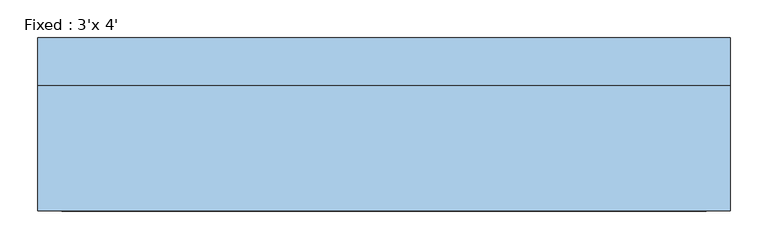
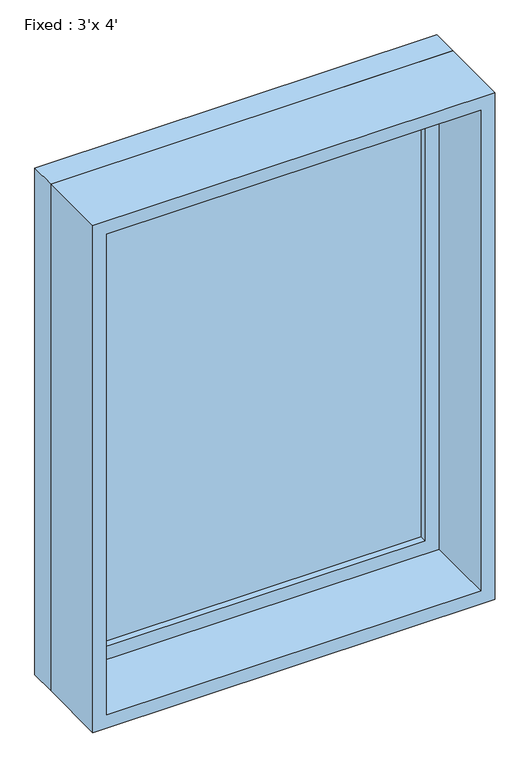
"""IFC4 building model written with IfcOpenShell, lengths in millimetres: window geometry, Fixed : 3'x 4'."""

from ifc_helpers import new_model, si_unit, frame, origin, place, context, project, spatial, polyline, outline, extrude, source, transform, mapped, element, save


def fixed_3_x_4_c1f32544(model_context):
    return source(origin(), model_context, "Body", "SweptSolid", [
        extrude(outline(polyline([(355.6, 66.675), (-431.8, 66.675), (-431.8, 79.375), (355.6, 79.375), (355.6, 66.675)])), frame((0.0, 0.0, 977.9), z_axis=(0.0, 0.0, 1.0), x_axis=(1.0, 0.0, 0.0)), (0.0, 0.0, 1.0), 1092.2),
        extrude(outline(polyline([(2114.55, -476.25), (933.45, -476.25), (933.45, 400.05), (2114.55, 400.05), (2114.55, -476.25)]), holes=[polyline([(2070.1, -431.8), (2070.1, 355.6), (977.9, 355.6), (977.9, -431.8), (2070.1, -431.8)])]), frame((0.0, 50.8, 0.0), z_axis=(0.0, 1.0, 0.0), x_axis=(0.0, 0.0, 1.0)), (0.0, 0.0, 1.0), 44.45),
        extrude(outline(polyline([(2133.6, -495.3), (914.4, -495.3), (914.4, 419.1), (2133.6, 419.1), (2133.6, -495.3)]), holes=[polyline([(2101.85, -463.55), (2101.85, 387.35), (946.15, 387.35), (946.15, -463.55), (2101.85, -463.55)])]), frame((0.0, -114.3, 0.0), z_axis=(0.0, 1.0, 0.0), x_axis=(0.0, 0.0, 1.0)), (0.0, 0.0, 1.0), 165.1),
        extrude(outline(polyline([(2133.6, 419.1), (2133.6, -495.3), (914.4, -495.3), (914.4, 419.1), (2133.6, 419.1)]), holes=[polyline([(2114.55, 400.05), (933.45, 400.05), (933.45, -476.25), (2114.55, -476.25), (2114.55, 400.05)])]), frame((0.0, 50.8, 0.0), z_axis=(0.0, 1.0, 0.0), x_axis=(0.0, 0.0, 1.0)), (0.0, 0.0, 1.0), 63.5),
    ])


if __name__ == "__main__":
    model = new_model("IFC4")
    model_context = context("Model", 3, world=origin())
    ifc_project = project(units=[si_unit("LENGTHUNIT", "METRE", prefix="MILLI")], contexts=[model_context])
    site = spatial("IfcSite", under=ifc_project)
    building = spatial("IfcBuilding", under=site)
    placement = place(None, origin())
    fixed_3_x_4_shape = fixed_3_x_4_c1f32544(model_context)
    element("IfcWindow", 1, ObjectType="Fixed : 3'x 4'", at=placement, inside=building, context=model_context, shape_type="MappedRepresentation", body=[
        mapped(fixed_3_x_4_shape, transform((0.0, 0.0, 0.0), x_axis=(1.0, 0.0, 0.0), y_axis=(0.0, 1.0, 0.0), z_axis=(0.0, 0.0, 1.0))),
    ])
    save(model, "model.ifc")

# Revit data of these elements
# Type "Fixed : 3'x 4'"
#   Type Mark = "18"
#   Construction Type Id = "GSP4R"
#   Assembly Code = "B2020100"
#   Analytic Construction = "1/8 in Pilkington single glazing"
#   Visual Light Transmittance = 0.9
#   Solar Heat Gain Coefficient = 0.78
#   Heat Transfer Coefficient (U) = 0.6496 BTU/(h·ft²·°F)
#   Height = 4' - 0"
#   Default Sill Height = 3' - 0"
#   Width = 3' - 0"
#   Window Inset = 0' - 0 3/4"
#   Define Thermal Properties by = 1
#   Glass Pane Material = Glass
#   Sash Material = Sash
#   Wall Closure = (empty or 0)
# Element 1 (IfcWindow, "Fixed : 3'x 4'")
#   Materials on its faces: "Sash", "Glass"
# Materials
#   "Glass": class "Glass", colour RGB 0 128 192, transparency 0.75, Description = "Soda Lime Glass", Cost = 0
#   "Sash": class "Wood", colour RGB 224 178 126, transparency 0, Cost = 0
